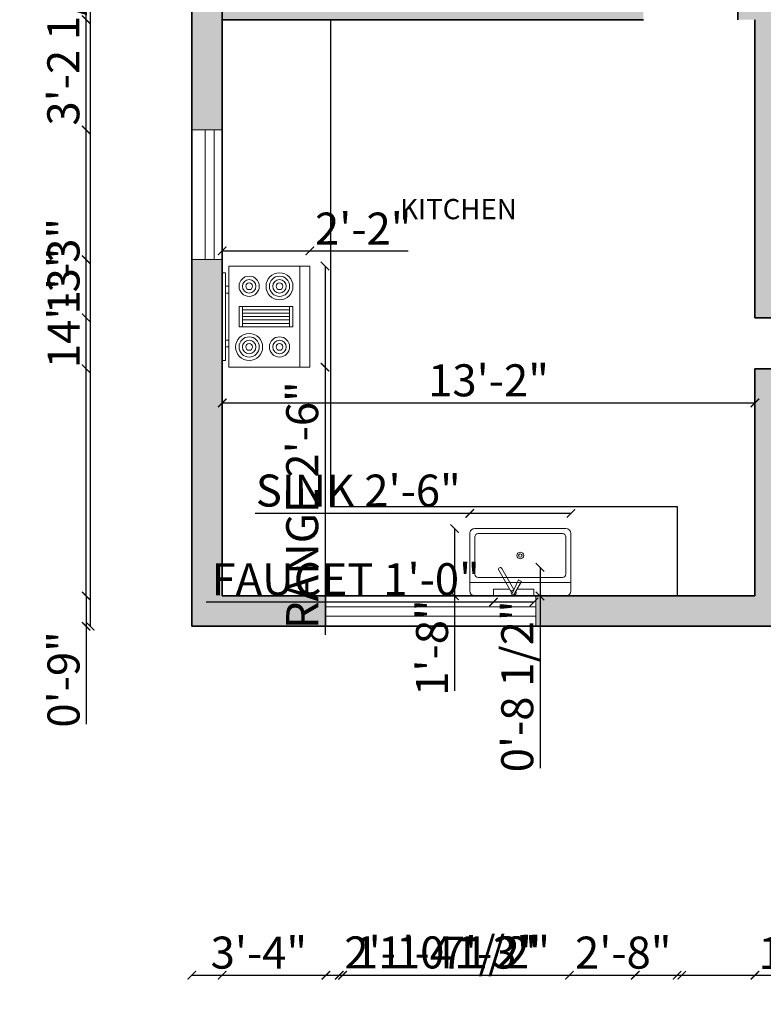
# Model space of a CAD drawing. Units: inches. Extents: x 1704 to 2334, y 1856 to 2559.
# Tile 1 of 10: x 1704 to 1925, y 1856 to 2148. Entities that reach past the tile are written whole.
import ezdxf

# ---------------------------------------------------------------- set-up
doc = ezdxf.new("R2010")
doc.units = ezdxf.units.IN
for name, color, linetype, lineweight in [('A-ANNO-DIMS', 2, 'Continuous', 18), ('A-AREA-IDEN', 7, 'Continuous', 18), ('A-EQPM', 8, 'Continuous', 18), ('A-FLOR-CASE', 32, 'Continuous', 25), ('A-FLOR-FIXT', 9, 'Continuous', 18), ('A-WALL', 7, 'Continuous', 35), ('WINDOW', 6, 'Continuous', 18)]:
    doc.layers.add(name, color=color, linetype=linetype, lineweight=lineweight)
doc.layers.add('A-WALL-PATT', color=18, linetype='Continuous', lineweight=13, true_color=0x000000)
doc.styles.get("Standard").update_dxf_attribs({"font": 'arial.ttf'})
doc.dimstyles.new('ISO-25', dxfattribs={"dimtxt": 9.5, "dimasz": 2.5, "dimexe": 1.25, "dimexo": 0.625, "dimtad": 1, "dimdec": 0, "dimlunit": 4, "dimtxsty": 'Standard', "dimblk": 'ARCHTICK', "dimcen": 2.5, "dimse1": 1, "dimse2": 1, "dimclrd": 3, "dimadec": 0, "dimazin": 0, "dimtfac": 1, "dimtdec": 0, "dimtmove": 0, "dimatfit": 3, "dimfxl": 1, "dimarcsym": 0})

# ---------------------------------------------------------------- blocks, each defined once
blk = doc.blocks.new('Range-Oven - 30 in top')
for p, q in [((0, -3), (30, -3)), ((12, -6), (18, -6)), ((13, -20), (13, -6)), ((14, -6), (14, -20)), ((15, -20), (15, -6)), ((16, -6), (16, -20)), ((17, -20), (17, -6)), ((18, -20), (12, -20)), ((6, -24), (6, -25)), ((8, -25), (8, -24)), ((22, -25), (22, -24)), ((24, -24), (24, -25))]:
    blk.add_line(p, q)
for points in [[(0, -24), (0, 0), (30, 0), (30, -24)], [(12, -21), (12, -5), (18, -5), (18, -21)], [(2, -26), (2, -25), (28, -25), (28, -26)]]:
    blk.add_lwpolyline(points, close=True)
for centre, radius in [((6, -9), 4), ((6, -9), 3), ((6, -9), 2), ((6, -9), 1), ((24, -9), 3), ((24, -9), 2), ((24, -9), 1), ((24, -18), 4), ((6, -18), 3), ((6, -18), 2), ((6, -18), 1), ((24, -18), 3), ((24, -18), 2), ((24, -18), 1)]:
    blk.add_circle(centre, radius)
blk = doc.blocks.new('Sink-single - 30 in top')
blk.add_line((-15, -3.999996), (15, -3.999996))
for points in [[(-13.5, 0), (13.5, 0)], [(-15, -18.499996), (-15, -1.5)], [(15, -1.5), (15, -18.499996)], [(-12.5, -5.499996), (12.5, -5.499996)], [(-13.5, -17.499996), (-13.5, -6.499996)], [(13.5, -6.499996), (13.5, -17.499996)], [(13.5, -19.999996), (-13.5, -19.999996)], [(12.5, -18.499996), (-12.5, -18.499996)]]:
    blk.add_lwpolyline(points)
for radius in [1, 0.5]:
    blk.add_circle((0, -11.999996), radius)
for centre, radius, start, end in [((-13.5, -1.5), 1.5, 90, 180), ((13.5, -1.5), 1.5, 0, 90), ((-12.5, -6.499996), 1, 90, 180), ((12.5, -6.499996), 1, 0, 90), ((-12.5, -17.499996), 1, 180, 270), ((12.5, -17.499996), 1, 270, 0), ((-13.5, -18.499996), 1.5, 180, 270), ((13.5, -18.499996), 1.5, 270, 0)]:
    blk.add_arc(centre, radius, start, end)
blk = doc.blocks.new('Faucet - single handle top')
for p, q in [((0.08, -0.26), (-2.26, -4.34)), ((-1.37, -4.79), (0.55, -0.5)), ((-0.06, -1.9), (3.57, -8.18)), ((4.43, -7.68), (0.72, -1.24)), ((-2.26, -4.34), (-1.37, -4.79))]:
    blk.add_line(p, q)
for points in [[(-0.92, -2), (-6, -2), (-6, 0), (6, 0), (6, -2), (1.16, -2)], [(-0.01, -2), (-0.12, -2)]]:
    blk.add_lwpolyline(points)
for centre, radius, start, end in [((0, -1), 0.75, 269.2246, 216.2304), ((4, -7.93), 0.5, 210, 30)]:
    blk.add_arc(centre, radius, start, end)
blk = doc.blocks.new('_ArchTick')
at = {"color": 0, "linetype": 'ByBlock', "const_width": 0.15}
blk.add_lwpolyline([(-0.5, -0.5), (0.5, 0.5)], dxfattribs=at)
blk = doc.blocks.new('*D20')
at = {"layer": 'A-ANNO-DIMS', "color": 0, "lineweight": -2, "transparency": 16777216}
blk.add_line((1764.01, 2034.32), (1922.01, 2034.32), dxfattribs=at)
at = {"layer": 'Defpoints', "color": 0, "transparency": 16777216}
for p in [(1922.01, 2034.32), (1764.01, 2027.85), (1922.01, 2027.85)]:
    blk.add_point(p, dxfattribs=at)
at = {"layer": 'A-ANNO-DIMS', "color": 0, "lineweight": -2, "transparency": 16777216, "xscale": 2.5, "yscale": 2.5, "zscale": 2.5, "rotation": 180}
blk.add_blockref('_ArchTick', (1764.01, 2034.32), dxfattribs=at)
at = {"layer": 'A-ANNO-DIMS', "color": 0, "lineweight": -2, "transparency": 16777216, "xscale": 2.5, "yscale": 2.5, "zscale": 2.5}
blk.add_blockref('_ArchTick', (1922.01, 2034.32), dxfattribs=at)
at = {"layer": 'A-ANNO-DIMS', "color": 0, "transparency": 16777216, "insert": (1843.01, 2039.8), "char_height": 9.5, "attachment_point": 5}
blk.add_mtext('13\'-2"', dxfattribs=at)
blk = doc.blocks.new('*D23')
at = {"layer": 'A-ANNO-DIMS', "color": 0, "lineweight": -2, "transparency": 16777216}
blk.add_line((1724.87, 2508.04), (1724.87, 1968.04), dxfattribs=at)
at = {"layer": 'Defpoints', "color": 0, "transparency": 16777216}
for p in [(1755.01, 2508.04), (1724.87, 1968.04), (1755.01, 1968.04)]:
    blk.add_point(p, dxfattribs=at)
at = {"layer": 'A-ANNO-DIMS', "color": 0, "lineweight": -2, "transparency": 16777216, "xscale": 2.5, "yscale": 2.5, "zscale": 2.5}
for p, rotation in [((1724.87, 2508.04), 90), ((1724.87, 1968.04), 270)]:
    blk.add_blockref('_ArchTick', p, dxfattribs=dict(at, rotation=rotation))
at = {"layer": 'A-ANNO-DIMS', "color": 0, "transparency": 16777216, "insert": (1719.41, 2238.04), "char_height": 9.5, "attachment_point": 5, "rotation": 90}
blk.add_mtext("45'", dxfattribs=at)
blk = doc.blocks.new('*D28')
at = {"layer": 'A-ANNO-DIMS', "color": 3, "lineweight": -2, "transparency": 16777216}
for p, q in [((1794.51, 2074.93), (1794.51, 2044.93)), ((1794.51, 2044.93), (1794.51, 1965.53))]:
    blk.add_line(p, q, dxfattribs=at)
at = {"layer": 'Defpoints', "color": 0, "transparency": 16777216}
for p in [(1790.01, 2074.93), (1790.01, 2044.93), (1794.51, 2044.93)]:
    blk.add_point(p, dxfattribs=at)
at = {"layer": 'A-ANNO-DIMS', "color": 3, "lineweight": -2, "transparency": 16777216, "xscale": 2.5, "yscale": 2.5, "zscale": 2.5}
for p, rotation in [((1794.51, 2074.93), 90), ((1794.51, 2044.93), 270)]:
    blk.add_blockref('_ArchTick', p, dxfattribs=dict(at, rotation=rotation))
at = {"layer": 'A-ANNO-DIMS', "color": 0, "transparency": 16777216, "insert": (1788.97, 2003.98), "char_height": 9.5, "attachment_point": 5, "rotation": 90}
blk.add_mtext('RANGE 2\'-6"', dxfattribs=at)
blk = doc.blocks.new('*D29')
at = {"layer": 'A-ANNO-DIMS', "color": 3, "lineweight": -2, "transparency": 16777216}
for p, q in [((1764.01, 2079.43), (1790.01, 2079.43)), ((1790.01, 2079.43), (1819.18, 2079.43))]:
    blk.add_line(p, q, dxfattribs=at)
at = {"layer": 'Defpoints', "color": 0, "transparency": 16777216}
for p in [(1790.01, 2079.43), (1764.01, 2074.93), (1790.01, 2074.93)]:
    blk.add_point(p, dxfattribs=at)
at = {"layer": 'A-ANNO-DIMS', "color": 3, "lineweight": -2, "transparency": 16777216, "xscale": 2.5, "yscale": 2.5, "zscale": 2.5, "rotation": 180}
blk.add_blockref('_ArchTick', (1764.01, 2079.43), dxfattribs=at)
at = {"layer": 'A-ANNO-DIMS', "color": 3, "lineweight": -2, "transparency": 16777216, "xscale": 2.5, "yscale": 2.5, "zscale": 2.5}
blk.add_blockref('_ArchTick', (1790.01, 2079.43), dxfattribs=at)
at = {"layer": 'A-ANNO-DIMS', "color": 0, "transparency": 16777216, "insert": (1805.84, 2084.82), "char_height": 9.5, "attachment_point": 5}
blk.add_mtext('2\'-2"', dxfattribs=at)
blk = doc.blocks.new('*D30')
at = {"layer": 'A-ANNO-DIMS', "color": 3, "lineweight": -2, "transparency": 16777216}
for p, q in [((1837.44, 2001.54), (1773.82, 2001.54)), ((1867.44, 2001.54), (1837.44, 2001.54))]:
    blk.add_line(p, q, dxfattribs=at)
at = {"layer": 'Defpoints', "color": 0, "transparency": 16777216}
for p in [(1837.44, 2001.54), (1837.44, 1997.04), (1867.44, 1997.04)]:
    blk.add_point(p, dxfattribs=at)
at = {"layer": 'A-ANNO-DIMS', "color": 3, "lineweight": -2, "transparency": 16777216, "xscale": 2.5, "yscale": 2.5, "zscale": 2.5, "rotation": 180}
blk.add_blockref('_ArchTick', (1837.44, 2001.54), dxfattribs=at)
at = {"layer": 'A-ANNO-DIMS', "color": 3, "lineweight": -2, "transparency": 16777216, "xscale": 2.5, "yscale": 2.5, "zscale": 2.5}
blk.add_blockref('_ArchTick', (1867.44, 2001.54), dxfattribs=at)
at = {"layer": 'A-ANNO-DIMS', "color": 0, "transparency": 16777216, "insert": (1804.38, 2007.08), "char_height": 9.5, "attachment_point": 5}
blk.add_mtext('SINK 2\'-6"', dxfattribs=at)
blk = doc.blocks.new('*D31')
at = {"layer": 'A-ANNO-DIMS', "color": 3, "lineweight": -2, "transparency": 16777216}
for p, q in [((1832.94, 1997.04), (1832.94, 1977.04)), ((1832.94, 1977.04), (1832.94, 1948.93))]:
    blk.add_line(p, q, dxfattribs=at)
at = {"layer": 'Defpoints', "color": 0, "transparency": 16777216}
for p in [(1837.44, 1997.04), (1832.94, 1977.04), (1837.44, 1977.04)]:
    blk.add_point(p, dxfattribs=at)
at = {"layer": 'A-ANNO-DIMS', "color": 3, "lineweight": -2, "transparency": 16777216, "xscale": 2.5, "yscale": 2.5, "zscale": 2.5}
for p, rotation in [((1832.94, 1997.04), 90), ((1832.94, 1977.04), 270)]:
    blk.add_blockref('_ArchTick', p, dxfattribs=dict(at, rotation=rotation))
at = {"layer": 'A-ANNO-DIMS', "color": 0, "transparency": 16777216, "insert": (1827.47, 1961.73), "char_height": 9.5, "attachment_point": 5, "rotation": 90}
blk.add_mtext('1\'-8"', dxfattribs=at)
blk = doc.blocks.new('*D32')
at = {"layer": 'A-ANNO-DIMS', "color": 3, "lineweight": -2, "transparency": 16777216}
for p, q in [((1844.49, 1975.24), (1759.26, 1975.24)), ((1856.49, 1975.24), (1844.49, 1975.24))]:
    blk.add_line(p, q, dxfattribs=at)
at = {"layer": 'Defpoints', "color": 0, "transparency": 16777216}
for p in [(1844.49, 1977.04), (1844.49, 1975.24), (1856.49, 1977.04)]:
    blk.add_point(p, dxfattribs=at)
at = {"layer": 'A-ANNO-DIMS', "color": 3, "lineweight": -2, "transparency": 16777216, "xscale": 2.5, "yscale": 2.5, "zscale": 2.5, "rotation": 180}
blk.add_blockref('_ArchTick', (1844.49, 1975.24), dxfattribs=at)
at = {"layer": 'A-ANNO-DIMS', "color": 3, "lineweight": -2, "transparency": 16777216, "xscale": 2.5, "yscale": 2.5, "zscale": 2.5}
blk.add_blockref('_ArchTick', (1856.49, 1975.24), dxfattribs=at)
at = {"layer": 'A-ANNO-DIMS', "color": 0, "transparency": 16777216, "insert": (1800.63, 1980.78), "char_height": 9.5, "attachment_point": 5}
blk.add_mtext('FAUCET 1\'-0"', dxfattribs=at)
blk = doc.blocks.new('*D33')
at = {"layer": 'A-ANNO-DIMS', "color": 3, "lineweight": -2, "transparency": 16777216}
for p, q in [((1858.29, 1985.54), (1858.29, 1977.04)), ((1858.29, 1977.04), (1858.29, 1925.9))]:
    blk.add_line(p, q, dxfattribs=at)
at = {"layer": 'Defpoints', "color": 0, "transparency": 16777216}
for p in [(1856.49, 1985.54), (1856.49, 1977.04), (1858.29, 1977.04)]:
    blk.add_point(p, dxfattribs=at)
at = {"layer": 'A-ANNO-DIMS', "color": 3, "lineweight": -2, "transparency": 16777216, "xscale": 2.5, "yscale": 2.5, "zscale": 2.5}
for p, rotation in [((1858.29, 1985.54), 90), ((1858.29, 1977.04), 270)]:
    blk.add_blockref('_ArchTick', p, dxfattribs=dict(at, rotation=rotation))
at = {"layer": 'A-ANNO-DIMS', "color": 0, "transparency": 16777216, "insert": (1852.76, 1950.22), "char_height": 9.5, "attachment_point": 5, "rotation": 90}
blk.add_mtext('0\'-8 1/2"', dxfattribs=at)
blk = doc.blocks.new('*D37')
at = {"layer": 'A-ANNO-DIMS', "color": 3, "lineweight": -2, "transparency": 16777216}
blk.add_line((1723.66, 1977.04), (1723.66, 2148.04), dxfattribs=at)
at = {"layer": 'Defpoints', "color": 0, "transparency": 16777216}
for p in [(1723.66, 2148.04), (1922.01, 2148.04), (1922.01, 1977.04)]:
    blk.add_point(p, dxfattribs=at)
at = {"layer": 'A-ANNO-DIMS', "color": 3, "lineweight": -2, "transparency": 16777216, "xscale": 2.5, "yscale": 2.5, "zscale": 2.5}
for p, rotation in [((1723.66, 2148.04), 90), ((1723.66, 1977.04), 270)]:
    blk.add_blockref('_ArchTick', p, dxfattribs=dict(at, rotation=rotation))
at = {"layer": 'A-ANNO-DIMS', "color": 0, "transparency": 16777216, "insert": (1718.18, 2062.54), "char_height": 9.5, "attachment_point": 5, "rotation": 90}
blk.add_mtext('14\'-3"', dxfattribs=at)
blk = doc.blocks.new('*D41')
at = {"layer": 'A-ANNO-DIMS', "color": 3, "lineweight": -2, "transparency": 16777216}
blk.add_line((1764.01, 1864.5), (1900.32, 1864.5), dxfattribs=at)
at = {"layer": 'Defpoints', "color": 0, "transparency": 16777216}
for p in [(1764.01, 2247.44), (1900.32, 2248.82), (1900.32, 1864.5)]:
    blk.add_point(p, dxfattribs=at)
at = {"layer": 'A-ANNO-DIMS', "color": 3, "lineweight": -2, "transparency": 16777216, "xscale": 2.5, "yscale": 2.5, "zscale": 2.5, "rotation": 180}
blk.add_blockref('_ArchTick', (1764.01, 1864.5), dxfattribs=at)
at = {"layer": 'A-ANNO-DIMS', "color": 3, "lineweight": -2, "transparency": 16777216, "xscale": 2.5, "yscale": 2.5, "zscale": 2.5}
blk.add_blockref('_ArchTick', (1900.32, 1864.5), dxfattribs=at)
at = {"layer": 'A-ANNO-DIMS', "color": 0, "transparency": 16777216, "insert": (1832.16, 1870.04), "char_height": 9.5, "attachment_point": 5}
blk.add_mtext('11\'-4 1/2"', dxfattribs=at)
blk = doc.blocks.new('*D43')
at = {"layer": 'A-ANNO-DIMS', "color": 3, "lineweight": -2, "transparency": 16777216}
blk.add_line((1764.01, 2539.39), (1796.13, 2539.39), dxfattribs=at)
at = {"layer": 'Defpoints', "color": 0, "transparency": 16777216}
for p in [(1796.13, 2539.39), (1764.01, 2148.04), (1796.13, 2148.04)]:
    blk.add_point(p, dxfattribs=at)
at = {"layer": 'A-ANNO-DIMS', "color": 3, "lineweight": -2, "transparency": 16777216, "xscale": 2.5, "yscale": 2.5, "zscale": 2.5, "rotation": 180}
blk.add_blockref('_ArchTick', (1764.01, 2539.39), dxfattribs=at)
at = {"layer": 'A-ANNO-DIMS', "color": 3, "lineweight": -2, "transparency": 16777216, "xscale": 2.5, "yscale": 2.5, "zscale": 2.5}
blk.add_blockref('_ArchTick', (1796.13, 2539.39), dxfattribs=at)
at = {"layer": 'A-ANNO-DIMS', "color": 0, "transparency": 16777216, "insert": (1780.07, 2544.86), "char_height": 9.5, "attachment_point": 5}
blk.add_mtext('2\'-8"', dxfattribs=at)
blk = doc.blocks.new('*D44')
at = {"layer": 'A-ANNO-DIMS', "color": 3, "lineweight": -2, "transparency": 16777216}
for p, q in [((2206.36, 2003.58), (2206.36, 2054.88)), ((2206.36, 1977.04), (2206.36, 2003.58))]:
    blk.add_line(p, q, dxfattribs=at)
at = {"layer": 'Defpoints', "color": 0, "transparency": 16777216}
for p in [(1898.93, 2003.58), (2206.36, 2003.58), (1898.93, 1977.04)]:
    blk.add_point(p, dxfattribs=at)
at = {"layer": 'A-ANNO-DIMS', "color": 3, "lineweight": -2, "transparency": 16777216, "xscale": 2.5, "yscale": 2.5, "zscale": 2.5}
for p, rotation in [((2206.36, 2003.58), 90), ((2206.36, 1977.04), 270)]:
    blk.add_blockref('_ArchTick', p, dxfattribs=dict(at, rotation=rotation))
at = {"layer": 'A-ANNO-DIMS', "color": 0, "transparency": 16777216, "insert": (2200.82, 2030.48), "char_height": 9.5, "attachment_point": 5, "rotation": 90}
blk.add_mtext('2\'-2 1/2"', dxfattribs=at)
blk = doc.blocks.new('*D45')
at = {"layer": 'A-ANNO-DIMS', "color": 3, "lineweight": -2, "transparency": 16777216}
for p, q in [((1898.93, 1864.5), (1922.01, 1864.5)), ((1922.01, 1864.5), (1957.5, 1864.5))]:
    blk.add_line(p, q, dxfattribs=at)
at = {"layer": 'Defpoints', "color": 0, "transparency": 16777216}
for p in [(1898.93, 1977.04), (1922.01, 1977.04), (1922.01, 1864.5)]:
    blk.add_point(p, dxfattribs=at)
at = {"layer": 'A-ANNO-DIMS', "color": 3, "lineweight": -2, "transparency": 16777216, "xscale": 2.5, "yscale": 2.5, "zscale": 2.5, "rotation": 180}
blk.add_blockref('_ArchTick', (1898.93, 1864.5), dxfattribs=at)
at = {"layer": 'A-ANNO-DIMS', "color": 3, "lineweight": -2, "transparency": 16777216, "xscale": 2.5, "yscale": 2.5, "zscale": 2.5}
blk.add_blockref('_ArchTick', (1922.01, 1864.5), dxfattribs=at)
at = {"layer": 'A-ANNO-DIMS', "color": 0, "transparency": 16777216, "insert": (1941, 1869.9), "char_height": 9.5, "attachment_point": 5}
blk.add_mtext('1\'-11"', dxfattribs=at)
blk = doc.blocks.new('*D53')
at = {"layer": 'A-ANNO-DIMS', "color": 3, "lineweight": -2, "transparency": 16777216}
for p, q in [((1764.01, 1864.5), (1798.75, 1864.5)), ((1798.75, 1864.5), (1857.43, 1864.5))]:
    blk.add_line(p, q, dxfattribs=at)
at = {"layer": 'Defpoints', "color": 0, "transparency": 16777216}
for p in [(1764.01, 2499.04), (1798.75, 2499.04), (1798.75, 1864.5)]:
    blk.add_point(p, dxfattribs=at)
at = {"layer": 'A-ANNO-DIMS', "color": 3, "lineweight": -2, "transparency": 16777216, "xscale": 2.5, "yscale": 2.5, "zscale": 2.5, "rotation": 180}
blk.add_blockref('_ArchTick', (1764.01, 1864.5), dxfattribs=at)
at = {"layer": 'A-ANNO-DIMS', "color": 3, "lineweight": -2, "transparency": 16777216, "xscale": 2.5, "yscale": 2.5, "zscale": 2.5}
blk.add_blockref('_ArchTick', (1798.75, 1864.5), dxfattribs=at)
at = {"layer": 'A-ANNO-DIMS', "color": 0, "transparency": 16777216, "insert": (1829.34, 1870.04), "char_height": 9.5, "attachment_point": 5}
blk.add_mtext('2\'-10 1/2"', dxfattribs=at)
blk = doc.blocks.new('*D59')
at = {"layer": 'A-ANNO-DIMS', "color": 3, "lineweight": -2, "transparency": 16777216}
for p, q in [((1723.66, 2115.31), (1723.66, 2166.44)), ((1723.66, 2076.84), (1723.66, 2115.31))]:
    blk.add_line(p, q, dxfattribs=at)
at = {"layer": 'Defpoints', "color": 0, "transparency": 16777216}
for p in [(1723.66, 2115.31), (1755.01, 2115.31), (1755.01, 2076.84)]:
    blk.add_point(p, dxfattribs=at)
at = {"layer": 'A-ANNO-DIMS', "color": 3, "lineweight": -2, "transparency": 16777216, "xscale": 2.5, "yscale": 2.5, "zscale": 2.5}
for p, rotation in [((1723.66, 2115.31), 90), ((1723.66, 2076.84), 270)]:
    blk.add_blockref('_ArchTick', p, dxfattribs=dict(at, rotation=rotation))
at = {"layer": 'A-ANNO-DIMS', "color": 0, "transparency": 16777216, "insert": (1718.12, 2142.12), "char_height": 9.5, "attachment_point": 5, "rotation": 90}
blk.add_mtext('3\'-2 1/2"', dxfattribs=at)
blk = doc.blocks.new('*D60')
at = {"layer": 'A-ANNO-DIMS', "color": 3, "lineweight": -2, "transparency": 16777216}
for p, q in [((1723.66, 2153.04), (1723.66, 2204.17)), ((1723.66, 2115.31), (1723.66, 2153.04))]:
    blk.add_line(p, q, dxfattribs=at)
at = {"layer": 'Defpoints', "color": 0, "transparency": 16777216}
for p in [(1723.66, 2153.04), (1764.01, 2153.04), (1755.01, 2115.31)]:
    blk.add_point(p, dxfattribs=at)
at = {"layer": 'A-ANNO-DIMS', "color": 3, "lineweight": -2, "transparency": 16777216, "xscale": 2.5, "yscale": 2.5, "zscale": 2.5}
for p, rotation in [((1723.66, 2153.04), 90), ((1723.66, 2115.31), 270)]:
    blk.add_blockref('_ArchTick', p, dxfattribs=dict(at, rotation=rotation))
at = {"layer": 'A-ANNO-DIMS', "color": 0, "transparency": 16777216, "insert": (1718.12, 2179.86), "char_height": 9.5, "attachment_point": 5, "rotation": 90}
blk.add_mtext('3\'-1 1/2"', dxfattribs=at)
blk = doc.blocks.new('*D61')
at = {"layer": 'A-ANNO-DIMS', "color": 3, "lineweight": -2, "transparency": 16777216}
blk.add_line((1755.01, 1864.5), (1794.77, 1864.5), dxfattribs=at)
at = {"layer": 'Defpoints', "color": 0, "transparency": 16777216}
for p in [(1755.01, 1968.04), (1794.77, 1968.04), (1794.77, 1864.5)]:
    blk.add_point(p, dxfattribs=at)
at = {"layer": 'A-ANNO-DIMS', "color": 3, "lineweight": -2, "transparency": 16777216, "xscale": 2.5, "yscale": 2.5, "zscale": 2.5, "rotation": 180}
blk.add_blockref('_ArchTick', (1755.01, 1864.5), dxfattribs=at)
at = {"layer": 'A-ANNO-DIMS', "color": 3, "lineweight": -2, "transparency": 16777216, "xscale": 2.5, "yscale": 2.5, "zscale": 2.5}
blk.add_blockref('_ArchTick', (1794.77, 1864.5), dxfattribs=at)
at = {"layer": 'A-ANNO-DIMS', "color": 0, "transparency": 16777216, "insert": (1774.89, 1869.98), "char_height": 9.5, "attachment_point": 5}
blk.add_mtext('3\'-4"', dxfattribs=at)
blk = doc.blocks.new('*D62')
at = {"layer": 'A-ANNO-DIMS', "color": 3, "lineweight": -2, "transparency": 16777216}
blk.add_line((1794.77, 2539.39), (1857.04, 2539.39), dxfattribs=at)
at = {"layer": 'Defpoints', "color": 0, "transparency": 16777216}
for p in [(1857.04, 2539.39), (1794.77, 1977.04), (1857.04, 1977.04)]:
    blk.add_point(p, dxfattribs=at)
at = {"layer": 'A-ANNO-DIMS', "color": 3, "lineweight": -2, "transparency": 16777216, "xscale": 2.5, "yscale": 2.5, "zscale": 2.5, "rotation": 180}
blk.add_blockref('_ArchTick', (1794.77, 2539.39), dxfattribs=at)
at = {"layer": 'A-ANNO-DIMS', "color": 3, "lineweight": -2, "transparency": 16777216, "xscale": 2.5, "yscale": 2.5, "zscale": 2.5}
blk.add_blockref('_ArchTick', (1857.04, 2539.39), dxfattribs=at)
at = {"layer": 'A-ANNO-DIMS', "color": 0, "transparency": 16777216, "insert": (1825.9, 2544.93), "char_height": 9.5, "attachment_point": 5}
blk.add_mtext('5\'-2 1/2"', dxfattribs=at)
blk = doc.blocks.new('*D65')
at = {"layer": 'A-ANNO-DIMS', "color": 3, "lineweight": -2, "transparency": 16777216}
for p, q in [((1723.66, 2059.61), (1723.66, 2087.72)), ((1723.66, 2044.47), (1723.66, 2059.61))]:
    blk.add_line(p, q, dxfattribs=at)
at = {"layer": 'Defpoints', "color": 0, "transparency": 16777216}
for p in [(1723.66, 2059.61), (1922.01, 2059.61), (1922.01, 2044.47)]:
    blk.add_point(p, dxfattribs=at)
at = {"layer": 'A-ANNO-DIMS', "color": 3, "lineweight": -2, "transparency": 16777216, "xscale": 2.5, "yscale": 2.5, "zscale": 2.5}
for p, rotation in [((1723.66, 2059.61), 90), ((1723.66, 2044.47), 270)]:
    blk.add_blockref('_ArchTick', p, dxfattribs=dict(at, rotation=rotation))
at = {"layer": 'A-ANNO-DIMS', "color": 0, "transparency": 16777216, "insert": (1718.18, 2074.92), "char_height": 9.5, "attachment_point": 5, "rotation": 90}
blk.add_mtext('1\'-3"', dxfattribs=at)
blk = doc.blocks.new('*D70')
at = {"layer": 'A-ANNO-DIMS', "color": 3, "lineweight": -2, "transparency": 16777216}
blk.add_line((1799.73, 1864.5), (1886.55, 1864.5), dxfattribs=at)
at = {"layer": 'Defpoints', "color": 0, "transparency": 16777216}
for p in [(1886.55, 2189.49), (1799.73, 2153.04), (1886.55, 1864.5)]:
    blk.add_point(p, dxfattribs=at)
at = {"layer": 'A-ANNO-DIMS', "color": 3, "lineweight": -2, "transparency": 16777216, "xscale": 2.5, "yscale": 2.5, "zscale": 2.5, "rotation": 180}
blk.add_blockref('_ArchTick', (1799.73, 1864.5), dxfattribs=at)
at = {"layer": 'A-ANNO-DIMS', "color": 3, "lineweight": -2, "transparency": 16777216, "xscale": 2.5, "yscale": 2.5, "zscale": 2.5}
blk.add_blockref('_ArchTick', (1886.55, 1864.5), dxfattribs=at)
at = {"layer": 'A-ANNO-DIMS', "color": 0, "transparency": 16777216, "insert": (1843.14, 1869.98), "char_height": 9.5, "attachment_point": 5}
blk.add_mtext('7\'-3"', dxfattribs=at)
blk = doc.blocks.new('*D76')
at = {"layer": 'A-ANNO-DIMS', "color": 3, "lineweight": -2, "transparency": 16777216}
for p, q in [((1723.66, 1977.04), (1723.66, 1968.04)), ((1723.66, 1968.04), (1723.66, 1939.04))]:
    blk.add_line(p, q, dxfattribs=at)
at = {"layer": 'Defpoints', "color": 0, "transparency": 16777216}
for p in [(1764.01, 1977.04), (1723.66, 1968.04), (1755.01, 1968.04)]:
    blk.add_point(p, dxfattribs=at)
at = {"layer": 'A-ANNO-DIMS', "color": 3, "lineweight": -2, "transparency": 16777216, "xscale": 2.5, "yscale": 2.5, "zscale": 2.5}
for p, rotation in [((1723.66, 1977.04), 90), ((1723.66, 1968.04), 270)]:
    blk.add_blockref('_ArchTick', p, dxfattribs=dict(at, rotation=rotation))
at = {"layer": 'A-ANNO-DIMS', "color": 0, "transparency": 16777216, "insert": (1718.18, 1952.29), "char_height": 9.5, "attachment_point": 5, "rotation": 90}
blk.add_mtext('0\'-9"', dxfattribs=at)
blk = doc.blocks.new('*D81')
at = {"layer": 'A-ANNO-DIMS', "color": 3, "lineweight": -2, "transparency": 16777216}
blk.add_line((2206.36, 2074.93), (2206.36, 2148.04), dxfattribs=at)
at = {"layer": 'Defpoints', "color": 0, "transparency": 16777216}
for p in [(1796.13, 2148.04), (2206.36, 2148.04), (1790.01, 2074.93)]:
    blk.add_point(p, dxfattribs=at)
at = {"layer": 'A-ANNO-DIMS', "color": 3, "lineweight": -2, "transparency": 16777216, "xscale": 2.5, "yscale": 2.5, "zscale": 2.5}
for p, rotation in [((2206.36, 2148.04), 90), ((2206.36, 2074.93), 270)]:
    blk.add_blockref('_ArchTick', p, dxfattribs=dict(at, rotation=rotation))
at = {"layer": 'A-ANNO-DIMS', "color": 0, "transparency": 16777216, "insert": (2200.88, 2111.48), "char_height": 9.5, "attachment_point": 5, "rotation": 90}
blk.add_mtext('6\'-1"', dxfattribs=at)
blk = doc.blocks.new('*D82')
at = {"layer": 'A-ANNO-DIMS', "color": 3, "lineweight": -2, "transparency": 16777216}
blk.add_line((1867, 1864.5), (1898.93, 1864.5), dxfattribs=at)
at = {"layer": 'Defpoints', "color": 0, "transparency": 16777216}
for p in [(1867, 1977.48), (1898.93, 1977.04), (1898.93, 1864.5)]:
    blk.add_point(p, dxfattribs=at)
at = {"layer": 'A-ANNO-DIMS', "color": 3, "lineweight": -2, "transparency": 16777216, "xscale": 2.5, "yscale": 2.5, "zscale": 2.5, "rotation": 180}
blk.add_blockref('_ArchTick', (1867, 1864.5), dxfattribs=at)
at = {"layer": 'A-ANNO-DIMS', "color": 3, "lineweight": -2, "transparency": 16777216, "xscale": 2.5, "yscale": 2.5, "zscale": 2.5}
blk.add_blockref('_ArchTick', (1898.93, 1864.5), dxfattribs=at)
at = {"layer": 'A-ANNO-DIMS', "color": 0, "transparency": 16777216, "insert": (1882.97, 1869.98), "char_height": 9.5, "attachment_point": 5}
blk.add_mtext('2\'-8"', dxfattribs=at)

msp = doc.modelspace()

# ---------------------------------------------------------------- hatches: boundary and pattern name
at = {"layer": 'A-WALL-PATT'}
h = msp.add_hatch(color=256, dxfattribs=at)
h.dxf.hatch_style = 1
h.paths.add_polyline_path([(1764.01, 2204.96), (1755.01, 2204.96), (1755.01, 2115.31), (1764.01, 2115.31)])
h.paths.add_polyline_path([(1764.01, 2076.84), (1755.01, 2076.84), (1755.01, 1968.04), (1794.77, 1968.04), (1794.77, 1977.04), (1764.01, 1977.04)])
h.paths.add_polyline_path([(1927.01, 1977.04), (1927.01, 2069.24), (1993.01, 2069.24), (1993.01, 1977.04)], flags=16)
h.paths.add_polyline_path([(1927.01, 2074.24), (1927.01, 2148.04), (1993.01, 2148.04), (1993.01, 2074.24)], flags=16)
h.paths.add_polyline_path([(1764.01, 2318.65), (1755.01, 2318.65), (1755.01, 2247.44), (1764.01, 2247.44)])
h.paths.add_polyline_path([(1764.01, 2499.04), (1798.75, 2499.04), (1798.75, 2508.04), (1755.01, 2508.04), (1755.01, 2336.43), (1764.01, 2336.43)])
h.paths.add_polyline_path([(1950.56, 2508.04), (1847.17, 2508.04), (1847.17, 2499.04), (1950.56, 2499.04)])
h.paths.add_polyline_path([(2059.64, 2508.04), (1975.68, 2508.04), (1975.68, 2499.04), (2059.64, 2499.04)])
h.paths.add_polyline_path([(2175.01, 2508.04), (2108.25, 2508.04), (2108.25, 2499.04), (2166.01, 2499.04), (2166.01, 1977.04), (2166.01, 1972.26), (2166.01, 1968.04), (2175.01, 1968.04)])
h.paths.add_polyline_path([(2166.01, 2319.04), (1993.01, 2319.04), (1993.01, 2273.04), (1998.01, 2273.04), (1998.01, 2314.04), (2166.01, 2314.04)])
h.paths.add_polyline_path([(2054.53, 2117.04), (1998.01, 2117.04), (1998.01, 2112.04), (2054.53, 2112.04)])
h.paths.add_polyline_path([(2166.01, 2117.04), (2105.53, 2117.04), (2105.53, 2112.04), (2166.01, 2112.04)])
h.paths.add_polyline_path([(1927.01, 2499.04), (1922.01, 2499.04), (1922.01, 2355.04), (1764.01, 2355.04), (1764.01, 2350.04), (1804.01, 2350.04), (1804.01, 2278.04), (1764.01, 2278.04), (1764.01, 2273.04), (1870.51, 2273.04), (1870.51, 2278.04), (1870.51, 2350.04), (1865.51, 2350.04), (1865.51, 2278.04), (1809.01, 2278.04), (1809.01, 2350.04), (1922.01, 2350.04), (1927.01, 2350.04), (1998.01, 2350.04), (1998.01, 2499.04), (1993.01, 2499.04), (1993.01, 2355.04), (1927.01, 2355.04)])
h.paths.add_polyline_path([(2131.1, 2203.36), (2144.85, 2203.36), (2144.85, 2212.38), (2131.1, 2212.38)], flags=25)
h.paths.add_polyline_path([(2010.94, 2265.21), (2036.85, 2265.21), (2036.85, 2274.23), (2010.94, 2274.23)], flags=9)
h.paths.add_polyline_path([(2010.9, 2274.71), (2056.95, 2274.71), (2056.95, 2284.04), (2010.9, 2284.04)], flags=25)
h.paths.add_polyline_path([(2003.27, 2440.18), (2049.79, 2440.18), (2049.79, 2449.51), (2003.27, 2449.51)], flags=9)
h.paths.add_polyline_path([(1934.96, 2428.22), (1967.48, 2428.22), (1967.48, 2437.55), (1934.96, 2437.55)], flags=25)
h.paths.add_polyline_path([(1778.93, 2466.23), (1827.79, 2466.23), (1827.79, 2475.56), (1778.93, 2475.56)], flags=25)
h.paths.add_polyline_path([(1938.32, 2043.05), (1970.37, 2043.05), (1970.37, 2052.39), (1938.32, 2052.39)], flags=8)
h.paths.add_polyline_path([(1932.21, 2095.38), (1956.75, 2095.38), (1956.75, 2104.56), (1932.21, 2104.56)], flags=8)
h.paths.add_polyline_path([(1888.97, 2148.04), (1888.97, 2153.04), (1764.01, 2153.04), (1764.01, 2148.04)])
h.paths.add_polyline_path([(1922.01, 2059.61), (1927.01, 2059.61), (1927.01, 2044.47), (1922.01, 2044.47), (1922.01, 1977.04), (1857.04, 1977.04), (1857.04, 1968.04), (1998.01, 1968.04), (1998.01, 1977.04), (1998.01, 2153.04), (1916.93, 2153.04), (1916.93, 2148.04), (1922.01, 2148.04)])

# ---------------------------------------------------------------- linework, layer by layer
at = {"layer": 'A-FLOR-CASE'}
for p, q in [((1796.13, 2148.04), (1796.13, 2003.58)), ((1796.13, 2003.58), (1898.93, 2003.58)), ((1898.93, 2003.58), (1898.93, 1977.04))]:
    msp.add_line(p, q, dxfattribs=at)
at = {"layer": 'A-WALL'}
for p, q in [((1764.01, 1977.04), (1764.01, 2499.04)), ((1916.93, 2153.04), (1916.93, 2148.04)), ((1764.01, 2148.04), (1888.97, 2148.04)), ((1922.01, 2059.61), (1922.01, 2148.04)), ((1927.01, 2059.61), (1922.01, 2059.61)), ((1922.01, 1977.04), (1922.01, 2044.47)), ((1927.01, 2044.47), (1922.01, 2044.47)), ((1922.01, 1977.04), (1764.01, 1977.04))]:
    msp.add_line(p, q, dxfattribs=at)
msp.add_lwpolyline([(1998.01, 1968.04), (1755.01, 1968.04), (1755.01, 2508.04), (2175.01, 2508.04), (2175.01, 1968.04), (2166.01, 1968.04)], dxfattribs=at)
at = {"layer": 'WINDOW'}
for p, q in [((1764.01, 2115.31), (1755.01, 2115.31)), ((1755.01, 2115.31), (1755.01, 2076.84)), ((1758.97, 2076.84), (1758.97, 2115.31)), ((1761.6, 2076.84), (1761.6, 2115.31)), ((1764.01, 2076.84), (1764.01, 2115.31)), ((1755.01, 2076.84), (1764.01, 2076.84)), ((1794.77, 1977.04), (1794.77, 1968.04)), ((1857.04, 1977.04), (1794.77, 1977.04)), ((1857.04, 1968.04), (1857.04, 1977.04)), ((1857.04, 1973.81), (1794.77, 1973.81)), ((1857.04, 1971.06), (1794.77, 1971.06)), ((1794.77, 1968.04), (1857.04, 1968.04))]:
    msp.add_line(p, q, dxfattribs=at)

# ---------------------------------------------------------------- block references
at = {"layer": 'A-EQPM', "rotation": 270}
msp.add_blockref('Range-Oven - 30 in top', (1790.01, 2074.93), dxfattribs=at)
at = {"layer": 'A-FLOR-FIXT', "rotation": 180}
for name, p in [('Sink-single - 30 in top', (1852.44, 1977.04)), ('Faucet - single handle top', (1850.49, 1977.04))]:
    msp.add_blockref(name, p, dxfattribs=at)

# ---------------------------------------------------------------- texts
at = {"layer": 'A-AREA-IDEN'}
msp.add_text('KITCHEN', height=6.013, dxfattribs=at).set_placement((1816.8, 2088.83))

# ---------------------------------------------------------------- dimensions: what is measured, and where the dimension line sits
at = {"layer": 'A-ANNO-DIMS'}
for base, p1, p2, override, picture, middle in [((1857.04, 2539.39), (1794.77, 1977.04), (1857.04, 1977.04), {"dimdec": 1, "dimlfac": 1, "dimrnd": 0, "dimzin": 1, "dimdsep": 46, "dimlunit": 4, "dimfrac": 2}, '*D62', (1825.9, 2544.93)), ((1796.13, 2539.39), (1764.01, 2148.04), (1796.13, 2148.04), {"dimdec": 1, "dimlfac": 1, "dimrnd": 0, "dimzin": 1, "dimdsep": 46, "dimlunit": 4, "dimfrac": 2}, '*D43', (1780.07, 2544.86)), ((1798.75, 1864.5), (1764.01, 2499.04), (1798.75, 2499.04), {"dimdec": 1, "dimlfac": 1, "dimrnd": 0, "dimzin": 1, "dimdsep": 46, "dimlunit": 4, "dimfrac": 2}, '*D53', (1829.34, 1870.04)), ((1900.32, 1864.5), (1764.01, 2247.44), (1900.32, 2248.82), {"dimdec": 1, "dimlfac": 1, "dimrnd": 0, "dimzin": 1, "dimdsep": 46, "dimlunit": 4, "dimfrac": 2}, '*D41', (1832.16, 1870.04)), ((1886.55, 1864.5), (1799.73, 2153.04), (1886.55, 2189.49), {"dimdec": 1, "dimlfac": 1, "dimrnd": 0, "dimzin": 1, "dimdsep": 46, "dimlunit": 4, "dimfrac": 2}, '*D70', (1843.14, 1869.98)), ((1790.01, 2079.43), (1764.01, 2074.93), (1790.01, 2074.93), {"dimdec": 1, "dimlfac": 1, "dimrnd": 0, "dimzin": 1, "dimdsep": 46, "dimlunit": 4, "dimfrac": 2}, '*D29', (1805.84, 2084.82)), ((1922.01, 2034.32), (1764.01, 2027.85), (1922.01, 2027.85), {"dimclrd": 0, "dimclre": 0, "dimclrt": 0}, '*D20', (1843.01, 2039.8)), ((1898.93, 1864.5), (1867, 1977.48), (1898.93, 1977.04), {"dimdec": 1, "dimlfac": 1, "dimrnd": 0, "dimzin": 1, "dimdsep": 46, "dimlunit": 4, "dimfrac": 2}, '*D82', (1882.97, 1869.98)), ((1922.01, 1864.5), (1898.93, 1977.04), (1922.01, 1977.04), {"dimdec": 1, "dimlfac": 1, "dimrnd": 0, "dimzin": 1, "dimdsep": 46, "dimlunit": 4, "dimfrac": 2}, '*D45', (1941, 1869.9)), ((1794.77, 1864.5), (1755.01, 1968.04), (1794.77, 1968.04), {"dimdec": 1, "dimlfac": 1, "dimrnd": 0, "dimzin": 1, "dimdsep": 46, "dimlunit": 4, "dimfrac": 2}, '*D61', (1774.89, 1869.98))]:
    dim = msp.add_linear_dim(base=base, p1=p1, p2=p2, dimstyle='ISO-25', override=override, dxfattribs=at)
    dim.commit()
    dim.dimension.update_dxf_attribs({"geometry": picture, "text_midpoint": middle})
for base, p1, p2, angle, override, picture, middle in [((1724.87, 1968.04), (1755.01, 2508.04), (1755.01, 1968.04), 90, {"dimclrd": 0, "dimclre": 0, "dimclrt": 0}, '*D23', (1719.41, 2238.04)), ((1723.66, 2153.04), (1755.01, 2115.31), (1764.01, 2153.04), 90, {"dimdec": 1, "dimlfac": 1, "dimrnd": 0, "dimzin": 1, "dimdsep": 46, "dimlunit": 4, "dimfrac": 2}, '*D60', (1718.12, 2179.86)), ((1723.66, 2115.31), (1755.01, 2076.84), (1755.01, 2115.31), 90, {"dimdec": 1, "dimlfac": 1, "dimrnd": 0, "dimzin": 1, "dimdsep": 46, "dimlunit": 4, "dimfrac": 2}, '*D59', (1718.12, 2142.12)), ((1723.66, 2148.04), (1922.01, 1977.04), (1922.01, 2148.04), 90, {"dimdec": 1, "dimlfac": 1, "dimrnd": 0, "dimzin": 1, "dimdsep": 46, "dimlunit": 4, "dimfrac": 2}, '*D37', (1718.18, 2062.54)), ((2206.36, 2148.04), (1790.01, 2074.93), (1796.13, 2148.04), 90, {"dimdec": 1, "dimlfac": 1, "dimrnd": 0, "dimzin": 1, "dimdsep": 46, "dimlunit": 4, "dimfrac": 2}, '*D81', (2200.88, 2111.48)), ((1723.66, 2059.61), (1922.01, 2044.47), (1922.01, 2059.61), 90, {"dimdec": 1, "dimlfac": 1, "dimrnd": 0, "dimzin": 1, "dimdsep": 46, "dimlunit": 4, "dimfrac": 2}, '*D65', (1718.18, 2074.92)), ((2206.36, 2003.58), (1898.93, 1977.04), (1898.93, 2003.58), 90, {"dimdec": 1, "dimlfac": 1, "dimrnd": 0, "dimzin": 1, "dimdsep": 46, "dimlunit": 4, "dimfrac": 2}, '*D44', (2200.82, 2030.48)), ((1832.94, 1977.04), (1837.44, 1997.04), (1837.44, 1977.04), 270, {"dimdec": 1, "dimlfac": 1, "dimrnd": 0, "dimzin": 1, "dimdsep": 46, "dimlunit": 4, "dimfrac": 2}, '*D31', (1827.47, 1961.73)), ((1858.29, 1977.04), (1856.49, 1985.54), (1856.49, 1977.04), 270, {"dimdec": 1, "dimlfac": 1, "dimrnd": 0, "dimzin": 1, "dimdsep": 46, "dimlunit": 4, "dimfrac": 2}, '*D33', (1852.76, 1950.22)), ((1723.66, 1968.04), (1764.01, 1977.04), (1755.01, 1968.04), 90, {"dimdec": 1, "dimlfac": 1, "dimrnd": 0, "dimzin": 1, "dimdsep": 46, "dimlunit": 4, "dimfrac": 2}, '*D76', (1718.18, 1952.29))]:
    dim = msp.add_linear_dim(base=base, p1=p1, p2=p2, angle=angle, dimstyle='ISO-25', override=override, dxfattribs=at)
    dim.commit()
    dim.dimension.update_dxf_attribs({"geometry": picture, "text_midpoint": middle})
for base, p1, p2, angle, text, picture, middle in [((1794.51, 2044.93), (1790.01, 2074.93), (1790.01, 2044.93), 270, 'RANGE <>', '*D28', (1788.97, 2003.98)), ((1837.44, 2001.54), (1867.44, 1997.04), (1837.44, 1997.04), 180, 'SINK <>', '*D30', (1804.38, 2007.08)), ((1844.49, 1975.24), (1856.49, 1977.04), (1844.49, 1977.04), 180, 'FAUCET <>', '*D32', (1800.63, 1980.78))]:
    dim = msp.add_linear_dim(base=base, p1=p1, p2=p2, angle=angle, text=text, dimstyle='ISO-25', override={"dimdec": 1, "dimlfac": 1, "dimrnd": 0, "dimzin": 1, "dimdsep": 46, "dimlunit": 4, "dimfrac": 2}, dxfattribs=at)
    dim.commit()
    dim.dimension.update_dxf_attribs({"geometry": picture, "text_midpoint": middle})

doc.saveas('drawing.dxf')
